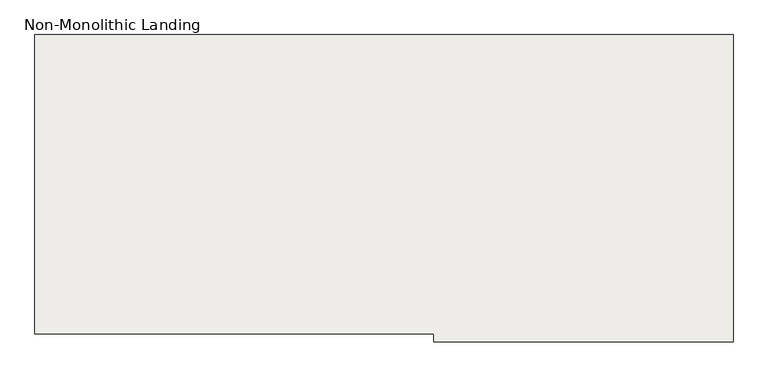
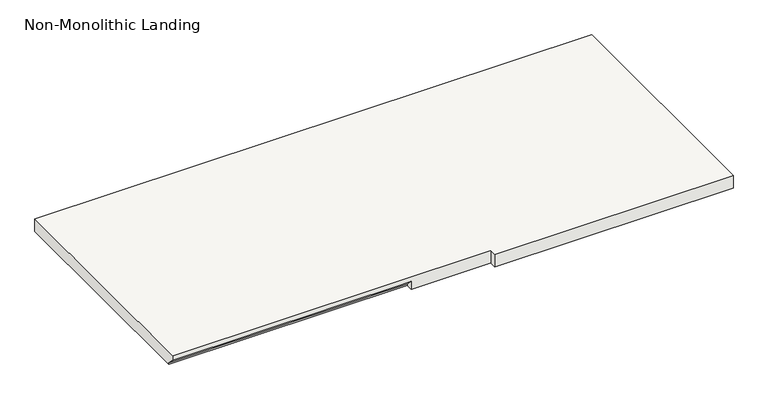
"""IFC4 building model written with IfcOpenShell, lengths in millimetres: slab geometry, Non-Monolithic Landing."""

from ifc_helpers import new_model, si_unit, origin, place, context, project, spatial, faceted_brep, source, transform, mapped, element, save


def non_monolithic_landing_d932be8a(model_context):
    return source(origin(), model_context, "Body", "Brep", [
        faceted_brep([(-3617.4415084, 23194.7216096, 42656.9005799), (-3617.4415084, 23220.1216096, 42631.5005799), (-2703.0415084, 23220.1216096, 42631.5005799), (-2703.0415084, 23194.7216096, 42656.9005799), (-2398.2415084, 23194.7216096, 42675.9505799), (-2398.2415084, 23169.3216096, 42675.9505799), (-1483.8415084, 23169.3216096, 42675.9505799), (-1483.8415084, 23194.7216096, 42675.9505799), (-1483.8415084, 24109.1216096, 42675.9505799), (-3617.4415084, 24109.1216096, 42675.9505799), (-3617.4415084, 23194.7216096, 42675.9505799), (-2703.0415084, 23220.1216096, 42625.1505799), (-3617.4415084, 23220.1216096, 42625.1505799), (-3617.4415084, 24109.1216096, 42625.1505799), (-1483.8415084, 24109.1216096, 42625.1505799), (-1483.8415084, 23194.7216096, 42625.1505799), (-1483.8415084, 23169.3216096, 42625.1505799), (-2398.2415084, 23169.3216096, 42625.1505799), (-2398.2415084, 23194.7216096, 42625.1505799), (-2703.0415084, 23194.7216096, 42625.1505799)], [[[0, 1, 2, 3]], [[4, 5, 6, 7, 8, 9, 10]], [[11, 12, 13, 14, 15, 16, 17, 18, 19]], [[12, 11, 2, 1]], [[11, 19, 3, 2]], [[4, 10, 0, 3, 19, 18]], [[5, 4, 18, 17]], [[6, 5, 17, 16]], [[7, 6, 16, 15]], [[8, 7, 15, 14]], [[9, 8, 14, 13]], [[10, 9, 13, 12, 1, 0]]]),
    ])


if __name__ == "__main__":
    model = new_model("IFC4")
    model_context = context("Model", 3, world=origin())
    ifc_project = project(units=[si_unit("LENGTHUNIT", "METRE", prefix="MILLI")], contexts=[model_context])
    site = spatial("IfcSite", under=ifc_project)
    building = spatial("IfcBuilding", under=site)
    placement = place(None, origin())
    non_monolithic_landing_shape = non_monolithic_landing_d932be8a(model_context)
    element("IfcSlab", 1, ObjectType="Non-Monolithic Landing", at=placement, inside=building, context=model_context, shape_type="MappedRepresentation", body=[
        mapped(non_monolithic_landing_shape, transform((0.0, 0.0, 0.0), x_axis=(1.0, 0.0, 0.0), y_axis=(0.0, 1.0, 0.0), z_axis=(0.0, 0.0, 1.0))),
    ])
    save(model, "model.ifc")
